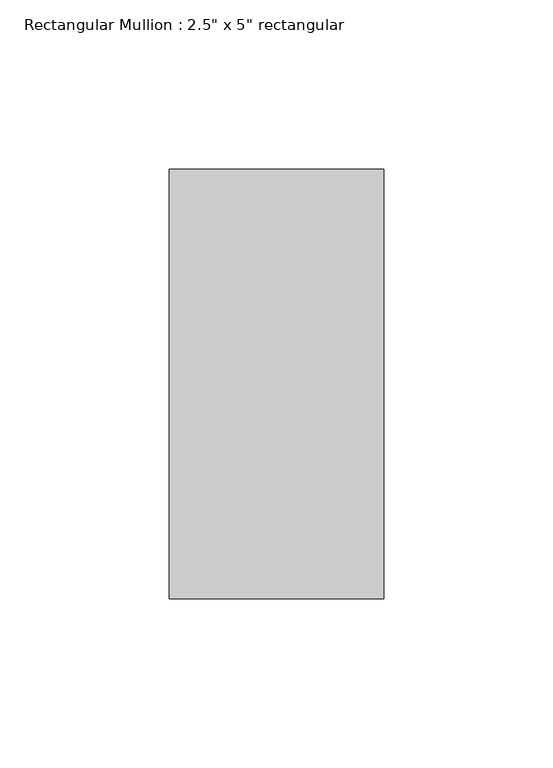
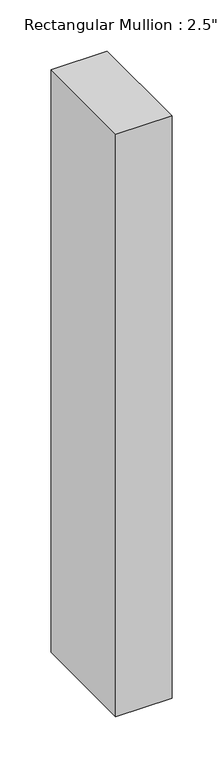
"""IFC4 building model written with IfcOpenShell, lengths in millimetres: member geometry."""

from ifc_helpers import new_model, si_unit, frame, origin, place, context, project, spatial, polyline, outline, extrude, source, transform, mapped, element, save


def member_802eba92(model_context):
    return source(origin(), model_context, "Body", "SweptSolid", [
        extrude(outline(polyline([(0.0, 63.5), (0.0, -63.5), (-63.5, -63.5), (-63.5, 63.5), (0.0, 63.5)])), frame((0.0, 0.0, -696.1594531), z_axis=(0.0, 0.0, 1.0), x_axis=(1.0, 0.0, 0.0)), (0.0, 0.0, 1.0), 696.1594531),
    ])


if __name__ == "__main__":
    model = new_model("IFC4")
    model_context = context("Model", 3, world=origin())
    ifc_project = project(units=[si_unit("LENGTHUNIT", "METRE", prefix="MILLI")], contexts=[model_context])
    site = spatial("IfcSite", under=ifc_project)
    building = spatial("IfcBuilding", under=site)
    placement = place(None, origin())
    member_shape = member_802eba92(model_context)
    element("IfcMember", 1, ObjectType="Rectangular Mullion : 2.5\" x 5\" rectangular", at=placement, inside=building, context=model_context, shape_type="MappedRepresentation", body=[
        mapped(member_shape, transform((0.0, 0.0, 0.0), x_axis=(1.0, 0.0, 0.0), y_axis=(0.0, 1.0, 0.0), z_axis=(0.0, 0.0, 1.0))),
    ])
    save(model, "model.ifc")

# Revit data of these elements
# Type "Rectangular Mullion : 2.5\" x 5\" rectangular"
#   built-in parameter 1007304 = 0.416667 (stored number, unit not read)
#   built-in parameter 1007301 = 0.104167 (stored number, unit not read)
#   built-in parameter 1007300 = 0.104167 (stored number, unit not read)
# Element 1 (IfcMember, "Rectangular Mullion : 2.5\" x 5\" rectangular")
#   Materials on its faces: "Aluminum"
# Materials
#   "Aluminum": class "Metal", colour RGB 247 247 247, transparency 0, Description = "Aluminum 6061", Cost = 0
